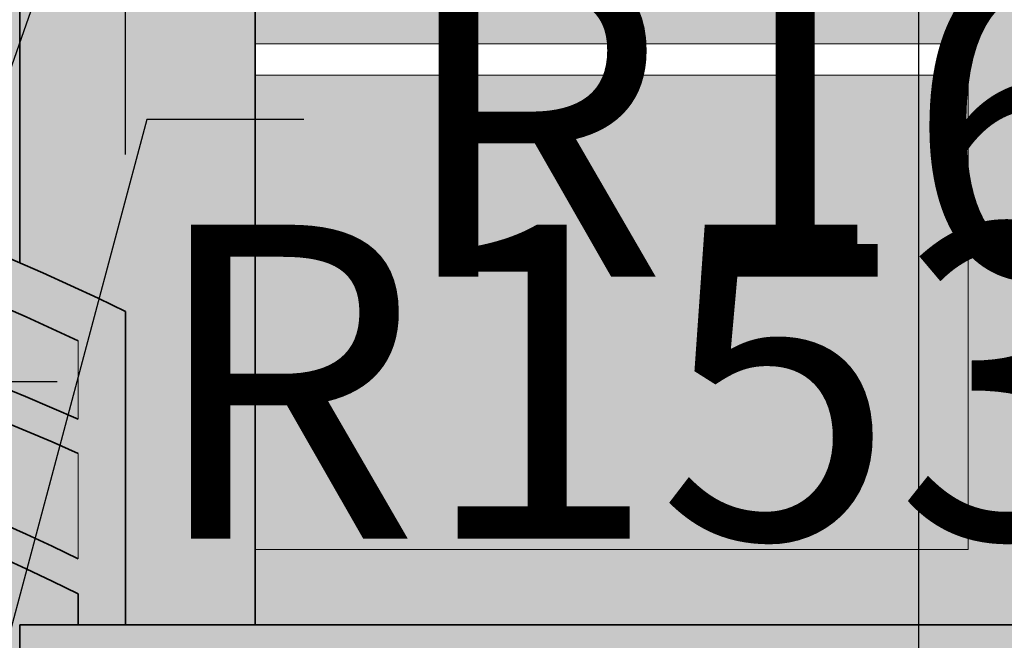
# Model space of a CAD drawing. Units: millimetres. Extents: x 130 to 1021, y 147 to 699.
# Tile 32 of 40: x 487 to 550, y 476 to 515. Entities that reach past the tile are written whole.
import ezdxf

# ---------------------------------------------------------------- set-up
doc = ezdxf.new("R2010")
doc.units = ezdxf.units.MM
doc.header["$MEASUREMENT"] = 0
for name, color, linetype, lineweight in [('A-ANNO-DIMS', 2, 'Continuous', 18), ('A-ELEV', 7, 'Continuous', 35), ('A-ELEV-PATT', 9, 'Continuous', 13), ('A-GLAZ', 4, 'Continuous', 18)]:
    doc.layers.add(name, color=color, linetype=linetype, lineweight=lineweight)
doc.styles.get("Standard").update_dxf_attribs({"font": 'arial.ttf'})
doc.dimstyles.get("Standard").update_dxf_attribs({"dimtxt": 20, "dimasz": 10, "dimexe": 10, "dimexo": 10, "dimgap": 5, "dimtad": 0, "dimtih": 1, "dimtoh": 1, "dimdec": 0, "dimzin": 0, "dimdsep": 46, "dimtxsty": 'Standard', "dimcen": 5, "dimadec": 0, "dimazin": 0, "dimtfac": 1, "dimtdec": 0, "dimtofl": 0, "dimtmove": 0, "dimatfit": 3, "dimfxl": 1, "dimtolj": 1, "dimtzin": 0, "dimarcsym": 0})

# ---------------------------------------------------------------- blocks, each defined once
blk = doc.blocks.new('*D11')
at = {"layer": 'A-ANNO-DIMS', "color": 0, "lineweight": -2, "transparency": 16777216}
for p, q in [((737.374, 648.699), (737.374, 149.739)), ((299.374, 566.947), (299.374, 149.739)), ((309.374, 159.739), (490.857, 159.739)), ((727.374, 159.739), (545.891, 159.739))]:
    blk.add_line(p, q, dxfattribs=at)
at = {"layer": 'A-ANNO-DIMS', "color": 0, "transparency": 16777216}
for points in [[(309.374, 161.406), (309.374, 158.073), (299.374, 159.739)], [(727.374, 161.406), (727.374, 158.073), (737.374, 159.739)]]:
    blk.add_solid(points, dxfattribs=at)
at = {"layer": 'Defpoints', "color": 0, "transparency": 16777216}
for p in [(737.374, 658.699), (299.374, 576.947), (737.374, 159.739)]:
    blk.add_point(p, dxfattribs=at)
at = {"layer": 'A-ANNO-DIMS', "color": 0, "transparency": 16777216, "insert": (518.374, 159.739), "char_height": 20, "attachment_point": 5}
blk.add_mtext('\\A1;438', dxfattribs=at)
blk = doc.blocks.new('*D12')
at = {"layer": 'A-ANNO-DIMS', "color": 0, "lineweight": -2, "transparency": 16777216}
for p, q in [((477.374, 661.947), (265.074, 661.947)), ((275.074, 651.947), (275.074, 438.205)), ((275.074, 194.039), (275.074, 407.782)), ((357.163, 184.039), (265.074, 184.039))]:
    blk.add_line(p, q, dxfattribs=at)
at = {"layer": 'A-ANNO-DIMS', "color": 0, "transparency": 16777216}
for points in [[(273.407, 651.947), (276.74, 651.947), (275.074, 661.947)], [(273.407, 194.039), (276.74, 194.039), (275.074, 184.039)]]:
    blk.add_solid(points, dxfattribs=at)
at = {"layer": 'Defpoints', "color": 0, "transparency": 16777216}
for p in [(275.074, 661.947), (487.374, 661.947), (367.163, 184.039)]:
    blk.add_point(p, dxfattribs=at)
at = {"layer": 'A-ANNO-DIMS', "color": 0, "transparency": 16777216, "insert": (275.074, 422.993), "char_height": 20, "attachment_point": 5}
blk.add_mtext('\\A1;477.9', dxfattribs=at)
blk = doc.blocks.new('*D19')
at = {"layer": 'A-ANNO-DIMS', "color": 0, "lineweight": -2, "transparency": 16777216}
for p, q in [((382.374, 388.947), (382.374, 696.247)), ((414.652, 510.881), (414.652, 696.247)), ((392.374, 686.247), (404.652, 686.247)), ((414.652, 686.247), (424.652, 686.247))]:
    blk.add_line(p, q, dxfattribs=at)
at = {"layer": 'A-ANNO-DIMS', "color": 0, "transparency": 16777216}
for points in [[(392.374, 687.914), (392.374, 684.581), (382.374, 686.247)], [(404.652, 687.914), (404.652, 684.581), (414.652, 686.247)]]:
    blk.add_solid(points, dxfattribs=at)
at = {"layer": 'Defpoints', "color": 0, "transparency": 16777216}
for p in [(414.652, 686.247), (414.652, 500.881), (382.374, 378.947)]:
    blk.add_point(p, dxfattribs=at)
at = {"layer": 'A-ANNO-DIMS', "color": 0, "transparency": 16777216, "insert": (463.411, 686.247), "char_height": 20, "attachment_point": 5}
blk.add_mtext('\\A1;32.28', dxfattribs=at)
blk = doc.blocks.new('*D20')
at = {"layer": 'A-ANNO-DIMS', "color": 0, "lineweight": -2, "transparency": 16777216}
for p, q in [((414.652, 510.881), (414.652, 696.247)), ((432.374, 388.947), (432.374, 696.247)), ((404.652, 686.247), (394.652, 686.247)), ((442.374, 686.247), (452.374, 686.247))]:
    blk.add_line(p, q, dxfattribs=at)
at = {"layer": 'A-ANNO-DIMS', "color": 0, "transparency": 16777216}
for points in [[(404.652, 687.914), (404.652, 684.581), (414.652, 686.247)], [(442.374, 687.914), (442.374, 684.581), (432.374, 686.247)]]:
    blk.add_solid(points, dxfattribs=at)
at = {"layer": 'Defpoints', "color": 0, "transparency": 16777216}
for p in [(432.374, 686.247), (414.652, 500.881), (432.374, 378.947)]:
    blk.add_point(p, dxfattribs=at)
at = {"layer": 'A-ANNO-DIMS', "color": 0, "transparency": 16777216, "insert": (490.075, 686.247), "char_height": 20, "attachment_point": 5}
blk.add_mtext('\\A1;17.72', dxfattribs=at)
blk = doc.blocks.new('*D21')
at = {"layer": 'A-ANNO-DIMS', "color": 0, "lineweight": -2, "transparency": 16777216}
for p, q in [((432.374, 388.947), (432.374, 696.247)), ((447.374, 656.947), (447.374, 696.247)), ((422.374, 686.247), (412.374, 686.247)), ((457.374, 686.247), (467.374, 686.247))]:
    blk.add_line(p, q, dxfattribs=at)
at = {"layer": 'A-ANNO-DIMS', "color": 0, "transparency": 16777216}
for points in [[(422.374, 687.914), (422.374, 684.581), (432.374, 686.247)], [(457.374, 687.914), (457.374, 684.581), (447.374, 686.247)]]:
    blk.add_solid(points, dxfattribs=at)
at = {"layer": 'Defpoints', "color": 0, "transparency": 16777216}
for p in [(447.374, 686.247), (447.374, 646.947), (432.374, 378.947)]:
    blk.add_point(p, dxfattribs=at)
at = {"layer": 'A-ANNO-DIMS', "color": 0, "transparency": 16777216, "insert": (485.832, 686.247), "char_height": 20, "attachment_point": 5}
blk.add_mtext('\\A1;15', dxfattribs=at)
blk = doc.blocks.new('*D22')
at = {"layer": 'A-ANNO-DIMS', "color": 0, "lineweight": -2, "transparency": 16777216}
for p, q in [((447.374, 656.947), (447.374, 696.247)), ((466.767, 403.947), (466.767, 696.247)), ((437.374, 686.247), (427.374, 686.247)), ((476.767, 686.247), (486.767, 686.247))]:
    blk.add_line(p, q, dxfattribs=at)
at = {"layer": 'A-ANNO-DIMS', "color": 0, "transparency": 16777216}
for points in [[(437.374, 687.914), (437.374, 684.581), (447.374, 686.247)], [(476.767, 687.914), (476.767, 684.581), (466.767, 686.247)]]:
    blk.add_solid(points, dxfattribs=at)
at = {"layer": 'Defpoints', "color": 0, "transparency": 16777216}
for p in [(466.767, 686.247), (447.374, 646.947), (466.767, 393.947)]:
    blk.add_point(p, dxfattribs=at)
at = {"layer": 'A-ANNO-DIMS', "color": 0, "transparency": 16777216, "insert": (532.34, 686.247), "char_height": 20, "attachment_point": 5}
blk.add_mtext('\\A1;19.393', dxfattribs=at)
blk = doc.blocks.new('*D23')
at = {"layer": 'A-ANNO-DIMS', "color": 0, "lineweight": -2, "transparency": 16777216}
for p, q in [((466.767, 403.947), (466.767, 696.247)), ((475.988, 209.039), (475.988, 696.247)), ((456.767, 686.247), (446.767, 686.247)), ((485.988, 686.247), (495.988, 686.247))]:
    blk.add_line(p, q, dxfattribs=at)
at = {"layer": 'A-ANNO-DIMS', "color": 0, "transparency": 16777216}
for points in [[(456.767, 687.914), (456.767, 684.581), (466.767, 686.247)], [(485.988, 687.914), (485.988, 684.581), (475.988, 686.247)]]:
    blk.add_solid(points, dxfattribs=at)
at = {"layer": 'Defpoints', "color": 0, "transparency": 16777216}
for p in [(475.988, 686.247), (466.767, 393.947), (475.988, 199.039)]:
    blk.add_point(p, dxfattribs=at)
at = {"layer": 'A-ANNO-DIMS', "color": 0, "transparency": 16777216, "insert": (534.631, 686.247), "char_height": 20, "attachment_point": 5}
blk.add_mtext('\\A1;9.222', dxfattribs=at)
blk = doc.blocks.new('*D24')
at = {"layer": 'A-ANNO-DIMS', "color": 0, "lineweight": -2, "transparency": 16777216}
for p, q in [((475.988, 209.039), (475.988, 696.247)), ((487.374, 671.947), (487.374, 696.247)), ((465.988, 686.247), (455.988, 686.247)), ((497.374, 686.247), (507.374, 686.247))]:
    blk.add_line(p, q, dxfattribs=at)
at = {"layer": 'A-ANNO-DIMS', "color": 0, "transparency": 16777216}
for points in [[(465.988, 687.914), (465.988, 684.581), (475.988, 686.247)], [(497.374, 687.914), (497.374, 684.581), (487.374, 686.247)]]:
    blk.add_solid(points, dxfattribs=at)
at = {"layer": 'Defpoints', "color": 0, "transparency": 16777216}
for p in [(487.374, 686.247), (487.374, 661.947), (475.988, 199.039)]:
    blk.add_point(p, dxfattribs=at)
at = {"layer": 'A-ANNO-DIMS', "color": 0, "transparency": 16777216, "insert": (553.022, 686.247), "char_height": 20, "attachment_point": 5}
blk.add_mtext('\\A1;11.385', dxfattribs=at)
blk = doc.blocks.new('*D25')
at = {"layer": 'A-ANNO-DIMS', "color": 0, "lineweight": -2, "transparency": 16777216}
for p, q in [((487.374, 671.947), (487.374, 696.247)), ((494.102, 506.908), (494.102, 696.247)), ((477.374, 686.247), (467.374, 686.247)), ((504.102, 686.247), (514.102, 686.247))]:
    blk.add_line(p, q, dxfattribs=at)
at = {"layer": 'A-ANNO-DIMS', "color": 0, "transparency": 16777216}
for points in [[(477.374, 687.914), (477.374, 684.581), (487.374, 686.247)], [(504.102, 687.914), (504.102, 684.581), (494.102, 686.247)]]:
    blk.add_solid(points, dxfattribs=at)
at = {"layer": 'Defpoints', "color": 0, "transparency": 16777216}
for p in [(494.102, 686.247), (487.374, 661.947), (494.102, 496.908)]:
    blk.add_point(p, dxfattribs=at)
at = {"layer": 'A-ANNO-DIMS', "color": 0, "transparency": 16777216, "insert": (552.922, 686.247), "char_height": 20, "attachment_point": 5}
blk.add_mtext('\\A1;6.728', dxfattribs=at)
blk = doc.blocks.new('*D26')
at = {"layer": 'A-ANNO-DIMS', "color": 0, "lineweight": -2, "transparency": 16777216}
for p, q in [((494.102, 506.908), (494.102, 696.247)), ((502.374, 593.947), (502.374, 696.247)), ((484.102, 686.247), (474.102, 686.247)), ((512.374, 686.247), (522.374, 686.247))]:
    blk.add_line(p, q, dxfattribs=at)
at = {"layer": 'A-ANNO-DIMS', "color": 0, "transparency": 16777216}
for points in [[(484.102, 687.914), (484.102, 684.581), (494.102, 686.247)], [(512.374, 687.914), (512.374, 684.581), (502.374, 686.247)]]:
    blk.add_solid(points, dxfattribs=at)
at = {"layer": 'Defpoints', "color": 0, "transparency": 16777216}
for p in [(502.374, 686.247), (502.374, 583.947), (494.102, 496.908)]:
    blk.add_point(p, dxfattribs=at)
at = {"layer": 'A-ANNO-DIMS', "color": 0, "transparency": 16777216, "insert": (561.03, 686.247), "char_height": 20, "attachment_point": 5}
blk.add_mtext('\\A1;8.272', dxfattribs=at)
blk = doc.blocks.new('*D27')
at = {"layer": 'A-ANNO-DIMS', "color": 0, "lineweight": -2, "transparency": 16777216}
for p, q in [((502.374, 593.947), (502.374, 696.247)), ((544.635, 396.264), (544.635, 696.247)), ((512.374, 686.247), (534.635, 686.247)), ((544.635, 686.247), (554.635, 686.247))]:
    blk.add_line(p, q, dxfattribs=at)
at = {"layer": 'A-ANNO-DIMS', "color": 0, "transparency": 16777216}
for points in [[(512.374, 687.914), (512.374, 684.581), (502.374, 686.247)], [(534.635, 687.914), (534.635, 684.581), (544.635, 686.247)]]:
    blk.add_solid(points, dxfattribs=at)
at = {"layer": 'Defpoints', "color": 0, "transparency": 16777216}
for p in [(544.635, 686.247), (502.374, 583.947), (544.635, 386.264)]:
    blk.add_point(p, dxfattribs=at)
at = {"layer": 'A-ANNO-DIMS', "color": 0, "transparency": 16777216, "insert": (593.776, 686.247), "char_height": 20, "attachment_point": 5}
blk.add_mtext('\\A1;42.26', dxfattribs=at)
blk = doc.blocks.new('*D28')
at = {"layer": 'A-ANNO-DIMS', "color": 0, "lineweight": -2, "transparency": 16777216}
for p, q in [((544.635, 396.264), (544.635, 696.247)), ((552.374, 593.947), (552.374, 696.247)), ((534.635, 686.247), (524.635, 686.247)), ((562.374, 686.247), (572.374, 686.247))]:
    blk.add_line(p, q, dxfattribs=at)
at = {"layer": 'A-ANNO-DIMS', "color": 0, "transparency": 16777216}
for points in [[(534.635, 687.914), (534.635, 684.581), (544.635, 686.247)], [(562.374, 687.914), (562.374, 684.581), (552.374, 686.247)]]:
    blk.add_solid(points, dxfattribs=at)
at = {"layer": 'Defpoints', "color": 0, "transparency": 16777216}
for p in [(552.374, 686.247), (552.374, 583.947), (544.635, 386.264)]:
    blk.add_point(p, dxfattribs=at)
at = {"layer": 'A-ANNO-DIMS', "color": 0, "transparency": 16777216, "insert": (611.057, 686.247), "char_height": 20, "attachment_point": 5}
blk.add_mtext('\\A1;7.738', dxfattribs=at)
blk = doc.blocks.new('*D54')
at = {"layer": 'A-ANNO-DIMS', "color": 0, "lineweight": -2, "transparency": 16777216}
for p, q in [((761.674, 473.947), (761.674, 483.947)), ((497.374, 463.947), (771.674, 463.947)), ((747.374, 403.69), (771.674, 403.69)), ((761.674, 393.69), (761.674, 383.69))]:
    blk.add_line(p, q, dxfattribs=at)
at = {"layer": 'A-ANNO-DIMS', "color": 0, "transparency": 16777216}
for points in [[(760.007, 473.947), (763.34, 473.947), (761.674, 463.947)], [(760.007, 393.69), (763.34, 393.69), (761.674, 403.69)]]:
    blk.add_solid(points, dxfattribs=at)
at = {"layer": 'Defpoints', "color": 0, "transparency": 16777216}
for p in [(487.374, 463.947), (761.674, 463.947), (737.374, 403.69)]:
    blk.add_point(p, dxfattribs=at)
at = {"layer": 'A-ANNO-DIMS', "color": 0, "transparency": 16777216, "insert": (761.674, 433.819), "char_height": 20, "attachment_point": 5}
blk.add_mtext('\\A1;60.26', dxfattribs=at)
blk = doc.blocks.new('*D55')
at = {"layer": 'A-ANNO-DIMS', "color": 0, "lineweight": -2, "transparency": 16777216}
for p, q in [((761.674, 486.947), (761.674, 496.947)), ((761.674, 496.947), (771.674, 496.947)), ((562.374, 476.947), (771.674, 476.947)), ((497.374, 463.947), (771.674, 463.947)), ((761.674, 453.947), (761.674, 443.947))]:
    blk.add_line(p, q, dxfattribs=at)
at = {"layer": 'A-ANNO-DIMS', "color": 0, "transparency": 16777216}
for points in [[(760.007, 486.947), (763.34, 486.947), (761.674, 476.947)], [(760.007, 453.947), (763.34, 453.947), (761.674, 463.947)]]:
    blk.add_solid(points, dxfattribs=at)
at = {"layer": 'Defpoints', "color": 0, "transparency": 16777216}
for p in [(552.374, 476.947), (761.674, 476.947), (487.374, 463.947)]:
    blk.add_point(p, dxfattribs=at)
at = {"layer": 'A-ANNO-DIMS', "color": 0, "transparency": 16777216, "insert": (790.057, 496.947), "char_height": 20, "attachment_point": 5}
blk.add_mtext('\\A1;13', dxfattribs=at)
blk = doc.blocks.new('*D65')
at = {"layer": 'A-ANNO-DIMS', "color": 0, "lineweight": -2, "transparency": 16777216}
for p, q in [((495.463, 509.127), (472.508, 423.108)), ((505.463, 509.127), (495.463, 509.127)), ((427.374, 248.979), (427.374, 258.979)), ((422.374, 253.979), (432.374, 253.979))]:
    blk.add_line(p, q, dxfattribs=at)
at = {"layer": 'A-ANNO-DIMS', "color": 0, "transparency": 16777216}
blk.add_solid([(470.898, 423.538), (474.118, 422.679), (469.93, 413.447)], dxfattribs=at)
at = {"layer": 'Defpoints', "color": 0, "transparency": 16777216}
for p in [(469.93, 413.447), (427.374, 253.979)]:
    blk.add_point(p, dxfattribs=at)
at = {"layer": 'A-ANNO-DIMS', "color": 0, "transparency": 16777216, "insert": (561.623, 509.127), "char_height": 20, "attachment_point": 5}
blk.add_mtext('\\A1;R165.05', dxfattribs=at)
blk = doc.blocks.new('*D67')
at = {"layer": 'A-ANNO-DIMS', "color": 0, "lineweight": -2, "transparency": 16777216}
for p, q in [((479.756, 492.431), (462.144, 412.223)), ((489.756, 492.431), (479.756, 492.431)), ((427.07, 247.496), (427.07, 257.496)), ((422.07, 252.496), (432.07, 252.496))]:
    blk.add_line(p, q, dxfattribs=at)
at = {"layer": 'A-ANNO-DIMS', "color": 0, "transparency": 16777216}
blk.add_solid([(460.516, 412.58), (463.772, 411.865), (459.999, 402.455)], dxfattribs=at)
at = {"layer": 'Defpoints', "color": 0, "transparency": 16777216}
for p in [(459.999, 402.455), (427.07, 252.496)]:
    blk.add_point(p, dxfattribs=at)
at = {"layer": 'A-ANNO-DIMS', "color": 0, "transparency": 16777216, "insert": (545.841, 492.431), "char_height": 20, "attachment_point": 5}
blk.add_mtext('\\A1;R153.53', dxfattribs=at)
blk = doc.blocks.new('*D69')
at = {"layer": 'A-ANNO-DIMS', "color": 0, "lineweight": -2, "transparency": 16777216}
for p, q in [((507.746, 572.261), (483.091, 501.813)), ((517.746, 572.261), (507.746, 572.261)), ((433.191, 354.23), (433.191, 364.23)), ((428.191, 359.23), (438.191, 359.23))]:
    blk.add_line(p, q, dxfattribs=at)
at = {"layer": 'A-ANNO-DIMS', "color": 0, "transparency": 16777216}
blk.add_solid([(481.518, 502.363), (484.664, 501.262), (479.788, 492.374)], dxfattribs=at)
at = {"layer": 'Defpoints', "color": 0, "transparency": 16777216}
for p in [(479.788, 492.374), (433.191, 359.23)]:
    blk.add_point(p, dxfattribs=at)
at = {"layer": 'A-ANNO-DIMS', "color": 0, "transparency": 16777216, "insert": (573.824, 572.261), "char_height": 20, "attachment_point": 5}
blk.add_mtext('\\A1;R141.06', dxfattribs=at)
blk = doc.blocks.new('*D71')
at = {"layer": 'A-ANNO-DIMS', "color": 0, "lineweight": -2, "transparency": 16777216}
for p, q in [((492.108, 581.609), (472.542, 512.666)), ((502.108, 581.609), (492.108, 581.609)), ((432.65, 367.109), (432.65, 377.109)), ((427.65, 372.109), (437.65, 372.109))]:
    blk.add_line(p, q, dxfattribs=at)
at = {"layer": 'A-ANNO-DIMS', "color": 0, "transparency": 16777216}
blk.add_solid([(470.938, 513.121), (474.145, 512.211), (469.812, 503.046)], dxfattribs=at)
at = {"layer": 'Defpoints', "color": 0, "transparency": 16777216}
for p in [(469.812, 503.046), (432.65, 372.109)]:
    blk.add_point(p, dxfattribs=at)
at = {"layer": 'A-ANNO-DIMS', "color": 0, "transparency": 16777216, "insert": (548.493, 581.609), "char_height": 20, "attachment_point": 5}
blk.add_mtext('\\A1;R136.1', dxfattribs=at)
blk = doc.blocks.new('*D72')
at = {"layer": 'A-ANNO-DIMS', "color": 0, "lineweight": -2, "transparency": 16777216}
for p, q in [((460.658, 573.64), (451.279, 503.49)), ((470.658, 573.64), (460.658, 573.64)), ((432.115, 355.142), (432.115, 365.142)), ((427.115, 360.142), (437.115, 360.142))]:
    blk.add_line(p, q, dxfattribs=at)
at = {"layer": 'A-ANNO-DIMS', "color": 0, "transparency": 16777216}
blk.add_solid([(449.628, 503.711), (452.931, 503.27), (449.954, 493.579)], dxfattribs=at)
at = {"layer": 'Defpoints', "color": 0, "transparency": 16777216}
for p in [(449.954, 493.579), (432.115, 360.142)]:
    blk.add_point(p, dxfattribs=at)
at = {"layer": 'A-ANNO-DIMS', "color": 0, "transparency": 16777216, "insert": (526.64, 573.64), "char_height": 20, "attachment_point": 5}
blk.add_mtext('\\A1;R134.62', dxfattribs=at)

msp = doc.modelspace()

# ---------------------------------------------------------------- hatches: boundary and pattern name
at = {"layer": 'A-ELEV-PATT'}
h = msp.add_hatch(color=256, dxfattribs=at)
h.dxf.hatch_style = 1
h.paths.add_polyline_path([(737.3738, 658.6988, 0.0135961), (632.4019, 661.9473), (607.3738, 661.9473), (487.3738, 661.9473), (487.3738, 649.9473), (607.3738, 649.9473), (632.3794, 649.9473, -0.0136841), (737.3738, 646.6784)])
h.paths.add_polyline_path([(732.3738, 643.9599, 0.0130529), (632.3738, 646.9473), (607.3738, 646.9473), (487.3738, 646.9473), (487.3738, 596.9473), (632.3738, 596.9473, -0.0130529), (732.3738, 593.9599)])
h.paths.add_polyline_path([(737.3738, 593.6732, 0.0137063), (632.3738, 596.9473), (487.3738, 596.9473), (487.3738, 586.9473), (632.355, 586.9473, -0.0137808), (737.3738, 583.6559)])
h.paths.add_polyline_path([(447.3738, 646.9473), (307.3738, 646.9473), (302.3738, 646.9473), (302.3738, 634.9473), (447.3738, 634.9473)])
h.paths.add_polyline_path([(447.3738, 631.9473), (307.3738, 631.9473), (307.3738, 586.9473), (447.3738, 586.9473)])
h.paths.add_polyline_path([(447.3738, 586.9473), (307.3738, 586.9473), (302.3738, 586.9473), (302.3738, 576.9473), (447.3738, 576.9473)])
h.paths.add_polyline_path([(447.3738, 573.9473), (367.3738, 573.9473), (367.3738, 539.9473), (447.3738, 539.9473)])
h.paths.add_polyline_path([(447.3738, 537.9473), (367.3738, 537.9473), (367.3738, 507.9473), (400.392, 507.4253, -0.001728), (401.3281, 507.6451, -0.5220025), (425.6117, 511.0391, -0.0391849), (447.3738, 510.4359), (447.3738, 510.7883)])
h.paths.add_polyline_path([(394.7238, 505.9473), (367.3738, 505.9473), (367.3738, 476.9473, -0.0146512), (375.8501, 480.2159), (376.1506, 499.2266, -0.0355419)])
h.paths.add_polyline_path([(632.3738, 583.9473), (552.3738, 583.9473), (552.3738, 550.9473), (632.3738, 550.9473)])
h.paths.add_polyline_path([(632.3738, 548.9473), (552.3738, 548.9473), (552.3738, 515.9473), (632.3738, 515.9473)])
h.paths.add_polyline_path([(632.3738, 513.9473), (552.3738, 513.9473), (552.3738, 476.9473), (632.3738, 476.9473)])
h.paths.add_polyline_path([(737.3738, 473.6903, 0.0136326), (632.3926, 476.9473), (552.3738, 476.9473), (487.3738, 476.9473), (487.3738, 466.9473), (632.3738, 466.9473, -0.0137063), (737.3738, 463.6732)])
h.paths.add_polyline_path([(732.3738, 460.9552, 0.0130741), (632.3681, 463.9473), (487.3738, 463.9473), (487.3738, 407.735, -0.0032286), (489.3544, 406.9473), (632.3926, 406.9473, -0.0129826), (732.3738, 403.9755)])
h.paths.add_polyline_path([(487.3738, 463.9473, 0.20133), (367.3738, 463.9473), (367.3738, 407.735, -0.1882031), (487.3738, 407.735)])
h.paths.add_polyline_path([(367.3738, 476.9473), (367.3738, 466.9473, -0.2013309), (487.3738, 466.9473), (487.3738, 476.9473, 0.20133)])
h.paths.add_polyline_path([(367.3738, 463.9473), (307.3738, 463.9473), (307.3738, 401.9473), (357.9413, 401.9473), (367.3738, 407.735)])
h.paths.add_polyline_path([(367.3738, 476.9473), (302.3738, 476.9473), (302.3738, 466.9473), (367.3738, 466.9473)])
h.paths.add_polyline_path([(632.8184, 366.9453), (552.3738, 366.9453), (552.3738, 393.9473), (632.8184, 393.9473)])
h.paths.add_polyline_path([(632.8184, 357.2114), (632.8184, 363.9453), (552.3738, 363.9453), (552.3738, 357.2114), (552.3738, 336.9453), (632.8184, 336.9453)])
h.paths.add_polyline_path([(632.8184, 333.9453), (552.3738, 333.9453), (552.3738, 306.9453), (632.8184, 306.9453)])
h.paths.add_polyline_path([(632.8184, 303.9453), (552.3738, 303.9453), (552.3738, 273.9473), (632.355, 273.9473, 0.0000608), (632.8184, 273.9491)])
h.paths.add_polyline_path([(737.3738, 403.6903, 0.0136326), (632.3926, 406.9473), (489.3544, 406.9473, 0.1915481), (367.3738, 407.735), (367.3738, 396.9473, -0.2013309), (487.3738, 396.9473), (632.3738, 396.9473, -0.0137063), (737.3738, 393.6732)])
h.paths.add_polyline_path([(357.9413, 401.9473), (307.3738, 401.9473), (307.3738, 391.9473), (357.9413, 391.9473)])
h.paths.add_polyline_path([(357.9413, 357.2114), (357.9413, 388.9473), (307.3738, 388.9473), (307.3738, 357.2114), (307.3738, 273.9473), (357.9413, 273.9473)])
h.paths.add_polyline_path([(732.3738, 263.93, -0.0130317), (632.3794, 260.9473), (466.7667, 260.9473), (466.7667, 240.9473), (469.8406, 236.978), (469.8406, 221.978), (472.9145, 218.0087), (472.9145, 213.9473), (607.3738, 213.9473), (732.3738, 213.9473)])
h.paths.add_polyline_path([(732.3738, 290.889), (722.479, 290.889), (722.479, 301.889), (732.3738, 301.889), (732.3738, 305.889), (722.479, 305.889), (722.479, 316.889), (732.3738, 316.889), (732.3738, 320.889), (722.479, 320.889), (722.479, 331.889), (732.3738, 331.889), (732.3738, 335.889), (722.479, 335.889), (722.479, 346.889), (732.3738, 346.889), (732.3738, 350.889), (722.479, 350.889), (722.479, 361.889), (732.3738, 361.889), (732.3738, 365.889), (722.479, 365.889), (722.479, 376.889), (732.3738, 376.889), (732.3738, 380.889), (722.479, 380.889), (722.479, 391.4848, 0.0005233), (718.479, 391.6843), (718.479, 380.889), (707.479, 380.889), (707.479, 392.1896, 0.0005231), (703.479, 392.3576), (703.479, 380.889), (692.479, 380.889), (692.479, 392.7765, 0.0005229), (688.479, 392.9131), (688.479, 380.889), (677.479, 380.889), (677.479, 393.2456, 0.0005228), (673.479, 393.3508), (673.479, 380.889), (662.479, 380.889), (662.479, 393.597, 0.0005227), (658.479, 393.6709), (658.479, 380.889), (647.479, 380.889), (647.479, 393.8308, 0.0005226), (643.479, 393.8732), (643.479, 380.889), (632.8184, 380.889), (632.8184, 376.889), (643.479, 376.889), (643.479, 365.889), (632.8184, 365.889), (632.8184, 361.889), (643.479, 361.889), (643.479, 350.889), (632.8184, 350.889), (632.8184, 346.889), (643.479, 346.889), (643.479, 335.889), (632.8184, 335.889), (632.8184, 331.889), (643.479, 331.889), (643.479, 320.889), (632.8184, 320.889), (632.8184, 316.889), (643.479, 316.889), (643.479, 305.889), (632.8184, 305.889), (632.8184, 301.889), (643.479, 301.889), (643.479, 290.889), (632.8184, 290.889), (632.8184, 286.889), (643.479, 286.889), (643.479, 274.0217, 0.0005246), (647.479, 274.0643), (647.479, 286.889), (658.479, 286.889), (658.479, 274.2248, 0.0005246), (662.479, 274.2989), (662.479, 286.889), (673.479, 286.889), (673.479, 274.546, 0.0005247), (677.479, 274.6516), (677.479, 286.889), (688.479, 286.889), (688.479, 274.9853, 0.0005248), (692.479, 275.1224), (692.479, 286.889), (703.479, 286.889), (703.479, 275.5429, 0.000525), (707.479, 275.7115), (707.479, 286.889), (718.479, 286.889), (718.479, 276.2187, 0.0005252), (722.479, 276.4189), (722.479, 286.889), (732.3738, 286.889)])
h.paths.add_polyline_path([(718.479, 290.889), (707.479, 290.889), (707.479, 301.889), (718.479, 301.889)], flags=16)
h.paths.add_polyline_path([(703.479, 290.889), (692.479, 290.889), (692.479, 301.889), (703.479, 301.889)], flags=16)
h.paths.add_polyline_path([(718.479, 305.889), (707.479, 305.889), (707.479, 316.889), (718.479, 316.889)], flags=16)
h.paths.add_polyline_path([(703.479, 305.889), (692.479, 305.889), (692.479, 316.889), (703.479, 316.889)], flags=16)
h.paths.add_polyline_path([(688.479, 290.889), (677.479, 290.889), (677.479, 301.889), (688.479, 301.889)], flags=16)
h.paths.add_polyline_path([(718.479, 320.889), (707.479, 320.889), (707.479, 331.889), (718.479, 331.889)], flags=16)
h.paths.add_polyline_path([(688.479, 305.889), (677.479, 305.889), (677.479, 316.889), (688.479, 316.889)], flags=16)
h.paths.add_polyline_path([(703.479, 320.889), (692.479, 320.889), (692.479, 331.889), (703.479, 331.889)], flags=16)
h.paths.add_polyline_path([(688.479, 320.889), (677.479, 320.889), (677.479, 331.889), (688.479, 331.889)], flags=16)
h.paths.add_polyline_path([(673.479, 290.889), (662.479, 290.889), (662.479, 301.889), (673.479, 301.889)], flags=16)
h.paths.add_polyline_path([(718.479, 335.889), (707.479, 335.889), (707.479, 346.889), (718.479, 346.889)], flags=16)
h.paths.add_polyline_path([(673.479, 305.889), (662.479, 305.889), (662.479, 316.889), (673.479, 316.889)], flags=16)
h.paths.add_polyline_path([(703.479, 335.889), (692.479, 335.889), (692.479, 346.889), (703.479, 346.889)], flags=16)
h.paths.add_polyline_path([(673.479, 320.889), (662.479, 320.889), (662.479, 331.889), (673.479, 331.889)], flags=16)
h.paths.add_polyline_path([(688.479, 335.889), (677.479, 335.889), (677.479, 346.889), (688.479, 346.889)], flags=16)
h.paths.add_polyline_path([(658.479, 290.889), (647.479, 290.889), (647.479, 301.889), (658.479, 301.889)], flags=16)
h.paths.add_polyline_path([(718.479, 350.889), (707.479, 350.889), (707.479, 361.889), (718.479, 361.889)], flags=16)
h.paths.add_polyline_path([(658.479, 305.889), (647.479, 305.889), (647.479, 316.889), (658.479, 316.889)], flags=16)
h.paths.add_polyline_path([(703.479, 350.889), (692.479, 350.889), (692.479, 361.889), (703.479, 361.889)], flags=16)
h.paths.add_polyline_path([(673.479, 335.889), (662.479, 335.889), (662.479, 346.889), (673.479, 346.889)], flags=16)
h.paths.add_polyline_path([(658.479, 320.889), (647.479, 320.889), (647.479, 331.889), (658.479, 331.889)], flags=16)
h.paths.add_polyline_path([(688.479, 350.889), (677.479, 350.889), (677.479, 361.889), (688.479, 361.889)], flags=16)
h.paths.add_polyline_path([(718.479, 365.889), (707.479, 365.889), (707.479, 376.889), (718.479, 376.889)], flags=16)
h.paths.add_polyline_path([(658.479, 335.889), (647.479, 335.889), (647.479, 346.889), (658.479, 346.889)], flags=16)
h.paths.add_polyline_path([(673.479, 350.889), (662.479, 350.889), (662.479, 361.889), (673.479, 361.889)], flags=16)
h.paths.add_polyline_path([(703.479, 365.889), (692.479, 365.889), (692.479, 376.889), (703.479, 376.889)], flags=16)
h.paths.add_polyline_path([(688.479, 365.889), (677.479, 365.889), (677.479, 376.889), (688.479, 376.889)], flags=16)
h.paths.add_polyline_path([(658.479, 350.889), (647.479, 350.889), (647.479, 361.889), (658.479, 361.889)], flags=16)
h.paths.add_polyline_path([(673.479, 365.889), (662.479, 365.889), (662.479, 376.889), (673.479, 376.889)], flags=16)
h.paths.add_polyline_path([(658.479, 365.889), (647.479, 365.889), (647.479, 376.889), (658.479, 376.889)], flags=16)
h.paths.add_polyline_path([(732.3738, 503.9786), (722.3392, 503.9786), (722.3392, 514.9786), (732.3738, 514.9786), (732.3738, 518.9786), (722.3392, 518.9786), (722.3392, 529.9786), (732.3738, 529.9786), (732.3738, 533.9786), (722.3392, 533.9786), (722.3392, 544.9786), (732.3738, 544.9786), (732.3738, 546.9473), (732.3738, 548.9786), (722.3392, 548.9786), (722.3392, 559.9786), (732.3738, 559.9786), (732.3738, 563.9786), (722.3392, 563.9786), (722.3392, 574.9786), (732.3738, 574.9786), (732.3738, 578.9786), (722.3392, 578.9786), (722.3392, 581.4789, 0.000526), (718.3392, 581.6791), (718.3392, 578.9786), (707.3392, 578.9786), (707.3392, 582.1863, 0.0005258), (703.3392, 582.355), (703.3392, 578.9786), (692.3392, 578.9786), (692.3392, 582.7752, 0.0005257), (688.3392, 582.9123), (688.3392, 578.9786), (677.3392, 578.9786), (677.3392, 583.2457, 0.0005255), (673.3392, 583.3512), (673.3392, 578.9786), (662.3392, 578.9786), (662.3392, 583.5978, 0.0005254), (658.3392, 583.6718), (658.3392, 578.9786), (647.3392, 578.9786), (647.3392, 583.8317, 0.0005254), (643.3392, 583.8741), (643.3392, 578.9786), (632.3738, 578.9786), (632.3738, 574.9786), (643.3392, 574.9786), (643.3392, 563.9786), (632.3738, 563.9786), (632.3738, 559.9786), (643.3392, 559.9786), (643.3392, 548.9786), (632.3738, 548.9786), (632.3738, 544.9786), (643.3392, 544.9786), (643.3392, 533.9786), (632.3738, 533.9786), (632.3738, 529.9786), (643.3392, 529.9786), (643.3392, 518.9786), (632.3738, 518.9786), (632.3738, 515.9473), (632.3738, 514.9786), (643.3392, 514.9786), (643.3392, 503.9786), (632.3738, 503.9786), (632.3738, 499.9786), (643.3392, 499.9786), (643.3392, 488.9786), (632.3738, 488.9786), (632.3738, 484.9786), (643.3392, 484.9786), (643.3392, 476.8751, -0.0005191), (647.3392, 476.8332), (647.3392, 484.9786), (658.3392, 484.9786), (658.3392, 476.6752, -0.0005192), (662.3392, 476.6022), (662.3392, 484.9786), (673.3392, 484.9786), (673.3392, 476.3585, -0.0005193), (677.3392, 476.2543), (677.3392, 484.9786), (688.3392, 484.9786), (688.3392, 475.9248, -0.0005194), (692.3392, 475.7894), (692.3392, 484.9786), (703.3392, 484.9786), (703.3392, 475.3741, -0.0005195), (707.3392, 475.2075), (707.3392, 484.9786), (718.3392, 484.9786), (718.3392, 474.7064, -0.0005197), (722.3392, 474.5086), (722.3392, 484.9786), (732.3738, 484.9786), (732.3738, 488.9786), (722.3392, 488.9786), (722.3392, 499.9786), (732.3738, 499.9786)])
h.paths.add_polyline_path([(718.3392, 503.9786), (707.3392, 503.9786), (707.3392, 514.9786), (718.3392, 514.9786)], flags=16)
h.paths.add_polyline_path([(718.3392, 499.9786), (718.3392, 488.9786), (707.3392, 488.9786), (707.3392, 499.9786)], flags=16)
h.paths.add_polyline_path([(718.3392, 518.9786), (707.3392, 518.9786), (707.3392, 529.9786), (718.3392, 529.9786)], flags=16)
h.paths.add_polyline_path([(703.3392, 503.9786), (692.3392, 503.9786), (692.3392, 514.9786), (703.3392, 514.9786)], flags=16)
h.paths.add_polyline_path([(703.3392, 499.9786), (703.3392, 488.9786), (692.3392, 488.9786), (692.3392, 499.9786)], flags=16)
h.paths.add_polyline_path([(703.3392, 518.9786), (692.3392, 518.9786), (692.3392, 529.9786), (703.3392, 529.9786)], flags=16)
h.paths.add_polyline_path([(718.3392, 533.9786), (707.3392, 533.9786), (707.3392, 544.9786), (718.3392, 544.9786)], flags=16)
h.paths.add_polyline_path([(688.3392, 503.9786), (677.3392, 503.9786), (677.3392, 514.9786), (688.3392, 514.9786)], flags=16)
h.paths.add_polyline_path([(688.3392, 499.9786), (688.3392, 488.9786), (677.3392, 488.9786), (677.3392, 499.9786)], flags=16)
h.paths.add_polyline_path([(703.3392, 533.9786), (692.3392, 533.9786), (692.3392, 544.9786), (703.3392, 544.9786)], flags=16)
h.paths.add_polyline_path([(688.3392, 518.9786), (677.3392, 518.9786), (677.3392, 529.9786), (688.3392, 529.9786)], flags=16)
h.paths.add_polyline_path([(688.3392, 533.9786), (677.3392, 533.9786), (677.3392, 544.9786), (688.3392, 544.9786)], flags=16)
h.paths.add_polyline_path([(718.3392, 548.9786), (707.3392, 548.9786), (707.3392, 559.9786), (718.3392, 559.9786)], flags=16)
h.paths.add_polyline_path([(673.3392, 503.9786), (662.3392, 503.9786), (662.3392, 514.9786), (673.3392, 514.9786)], flags=16)
h.paths.add_polyline_path([(673.3392, 499.9786), (673.3392, 488.9786), (662.3392, 488.9786), (662.3392, 499.9786)], flags=16)
h.paths.add_polyline_path([(703.3392, 548.9786), (692.3392, 548.9786), (692.3392, 559.9786), (703.3392, 559.9786)], flags=16)
h.paths.add_polyline_path([(673.3392, 518.9786), (662.3392, 518.9786), (662.3392, 529.9786), (673.3392, 529.9786)], flags=16)
h.paths.add_polyline_path([(688.3392, 548.9786), (677.3392, 548.9786), (677.3392, 559.9786), (688.3392, 559.9786)], flags=16)
h.paths.add_polyline_path([(673.3392, 533.9786), (662.3392, 533.9786), (662.3392, 544.9786), (673.3392, 544.9786)], flags=16)
h.paths.add_polyline_path([(718.3392, 563.9786), (707.3392, 563.9786), (707.3392, 574.9786), (718.3392, 574.9786)], flags=16)
h.paths.add_polyline_path([(658.3392, 503.9786), (647.3392, 503.9786), (647.3392, 514.9786), (658.3392, 514.9786)], flags=16)
h.paths.add_polyline_path([(658.3392, 499.9786), (658.3392, 488.9786), (647.3392, 488.9786), (647.3392, 499.9786)], flags=16)
h.paths.add_polyline_path([(703.3392, 563.9786), (692.3392, 563.9786), (692.3392, 574.9786), (703.3392, 574.9786)], flags=16)
h.paths.add_polyline_path([(658.3392, 518.9786), (647.3392, 518.9786), (647.3392, 529.9786), (658.3392, 529.9786)], flags=16)
h.paths.add_polyline_path([(673.3392, 548.9786), (662.3392, 548.9786), (662.3392, 559.9786), (673.3392, 559.9786)], flags=16)
h.paths.add_polyline_path([(688.3392, 563.9786), (677.3392, 563.9786), (677.3392, 574.9786), (688.3392, 574.9786)], flags=16)
h.paths.add_polyline_path([(658.3392, 533.9786), (647.3392, 533.9786), (647.3392, 544.9786), (658.3392, 544.9786)], flags=16)
h.paths.add_polyline_path([(673.3392, 563.9786), (662.3392, 563.9786), (662.3392, 574.9786), (673.3392, 574.9786)], flags=16)
h.paths.add_polyline_path([(658.3392, 548.9786), (647.3392, 548.9786), (647.3392, 559.9786), (658.3392, 559.9786)], flags=16)
h.paths.add_polyline_path([(658.3392, 563.9786), (647.3392, 563.9786), (647.3392, 574.9786), (658.3392, 574.9786)], flags=16)
h = msp.add_hatch(color=256, dxfattribs=at)
h.dxf.hatch_style = 1
h.paths.add_polyline_path([(447.3738, 576.9473), (302.3738, 576.9473), (302.3738, 573.9473), (447.3738, 573.9473)])
h.paths.add_polyline_path([(487.3738, 583.9473), (487.3738, 586.9473), (447.3738, 576.9473), (447.3738, 573.9473)])
h.paths.add_polyline_path([(632.355, 586.9473), (487.3738, 586.9473), (487.3738, 583.9473), (632.3738, 583.9473), (632.3738, 583.9472, -0.0138), (737.3738, 580.6507), (737.3738, 583.6559, 0.0137808)])
h.paths.add_polyline_path([(367.3738, 466.9473), (302.3738, 466.9473), (302.3738, 463.9473), (367.3738, 463.9473)])
h.paths.add_polyline_path([(487.3738, 463.9473), (487.3738, 466.9473, 0.2013309), (367.3738, 466.9473), (367.3738, 463.9473, -0.20133)])
h.paths.add_polyline_path([(632.3738, 466.9473), (487.3738, 466.9473), (487.3738, 463.9473), (632.3681, 463.9473, -0.0137285), (737.3738, 460.6681), (737.3738, 463.6732, 0.0137063)])
h.paths.add_polyline_path([(632.3738, 396.9473), (487.3738, 396.9473, 0.2013309), (367.3738, 396.9473), (367.3738, 393.9473, -0.2023717), (486.7667, 393.9473), (632.3681, 393.9473, -0.0137285), (737.3738, 390.6681), (737.3738, 393.6732, 0.0137063)])
h.paths.add_polyline_path([(357.9413, 391.9473), (307.3738, 391.9473), (307.3738, 388.9473), (357.9413, 388.9473)])
h.paths.add_polyline_path([(367.3738, 393.9473), (367.3738, 396.9473), (357.9413, 391.924), (357.9413, 388.9473), (358.058, 388.9473)])
h.paths.add_polyline_path([(737.3738, 264.2162), (737.3738, 267.2214, -0.0137063), (632.3738, 263.9473), (463.7667, 263.9473), (466.7667, 260.9473), (632.3794, 260.9473, 0.0136841)])
h.paths.add_polyline_path([(463.7667, 263.9473), (447.3738, 263.9473), (450.3738, 260.9473), (466.7667, 260.9473)])
h.paths.add_polyline_path([(447.3738, 263.9473), (432.3738, 263.9473), (432.3738, 260.9473), (450.3738, 260.9473)])
h.paths.add_polyline_path([(382.3738, 263.9473), (357.9413, 263.9473), (357.9413, 260.9473), (382.3738, 260.9473)])
h.paths.add_polyline_path([(357.9413, 263.9473), (307.3738, 263.9473), (307.3738, 260.9473), (357.9413, 260.9473)])
h = msp.add_hatch(color=256, dxfattribs=at)
h.paths.add_polyline_path([(327.3738, 569.884), (327.3738, 573.9473), (307.3738, 573.9473), (307.3738, 476.9473), (327.3738, 476.9473), (327.3738, 480.95)])
h.paths.add_polyline_path([(486.7667, 386.2639), (486.7667, 393.9473), (466.7667, 393.9473), (466.7667, 357.2114), (466.7667, 311.9335, 0.0342703), (486.7667, 308.4637)])
h.paths.add_polyline_path([(486.7667, 308.4637, -0.0342703), (466.7667, 311.9335), (466.7667, 273.9473), (486.7667, 273.9473)])
h.paths.add_polyline_path([(389.3738, 351.5473), (396.7693, 351.5473, -0.007027), (393.8774, 354.5473), (389.3738, 354.5473), (389.3738, 359.5775, -0.0190302), (382.3738, 368.424), (382.3738, 249.5473), (432.3738, 249.5473), (432.3738, 325.067, -0.0057673), (429.3738, 326.709), (429.3738, 257.5473), (426.3738, 257.5473), (426.3738, 328.4428, -0.0059254), (423.3738, 330.272), (423.3738, 315.7473), (389.3738, 315.7473), (389.3738, 332.1473), (420.4552, 332.1473, -0.008951), (416.0768, 335.1473), (389.3738, 335.1473)])
h.paths.add_polyline_path([(389.3738, 312.7473), (423.3738, 312.7473), (423.3738, 296.3473), (389.3738, 296.3473)], flags=16)
h.paths.add_polyline_path([(389.3738, 293.3473), (423.3738, 293.3473), (423.3738, 276.9473), (389.3738, 276.9473)], flags=16)
h.paths.add_polyline_path([(389.3738, 273.9473), (423.3738, 273.9473), (423.3738, 257.5473), (389.3738, 257.5473)], flags=16)
h.paths.add_polyline_path([(432.3738, 378.9473), (382.3738, 378.9473), (382.3738, 368.424, 0.0190302), (389.3738, 359.5775), (389.3738, 370.9473), (423.3738, 370.9473), (423.3738, 354.5473), (393.8774, 354.5473, 0.007027), (396.7693, 351.5473), (423.3738, 351.5473), (423.3738, 335.1473), (416.0768, 335.1473, 0.008951), (420.4552, 332.1473), (423.3738, 332.1473), (423.3738, 330.272, 0.0059254), (426.3738, 328.4428), (426.3738, 370.9473), (429.3738, 370.9473), (429.3738, 326.709, 0.0057673), (432.3738, 325.067)])
h.paths.add_polyline_path([(466.7667, 357.2114), (466.7667, 393.9473), (447.3738, 393.9473), (447.3738, 357.2114), (447.3738, 318.1243, 0.0063261), (450.8779, 316.785), (450.8779, 331.5915), (463.5608, 331.5915), (463.5608, 312.7571, 0.005582), (466.7667, 311.9335)])
h.paths.add_polyline_path([(450.8779, 334.5915), (450.8779, 360.0915), (463.5608, 360.0915), (463.5608, 334.5915)], flags=16)
h.paths.add_polyline_path([(450.8779, 363.0915), (450.8779, 388.6449), (463.5608, 388.6449), (463.5608, 363.0915)], flags=16)
h.paths.add_polyline_path([(466.7667, 311.9335, -0.005582), (463.5608, 312.7571), (463.5608, 306.0915), (450.8779, 306.0915), (450.8779, 316.785, -0.0063261), (447.3738, 318.1243), (447.3738, 273.9473), (466.7667, 273.9473)])
h.paths.add_polyline_path([(450.8779, 303.0915), (463.5608, 303.0915), (463.5608, 277.5915), (450.8779, 277.5915)], flags=16)
h.paths.add_polyline_path([(552.3738, 357.2114), (552.3738, 393.9473), (486.7667, 393.9473), (486.7667, 386.2639), (544.6354, 386.2639), (544.6354, 280.6619), (486.7667, 280.6619), (486.7667, 273.9473), (552.3738, 273.9473)])
h.paths.add_polyline_path([(487.3738, 583.9473), (472.3738, 580.1973), (472.3738, 507.0765), (472.3738, 505.4251, -0.0056452), (475.3738, 504.4942), (475.3738, 506.3543), (475.3738, 511.9473), (484.3738, 511.9473), (484.3738, 503.8134), (484.3738, 501.2439, -0.0058357), (487.3738, 500.0015)])
h.paths.add_polyline_path([(484.3738, 578.0434), (484.3738, 548.9473), (475.3738, 548.9473), (475.3738, 575.7934)], flags=16)
h.paths.add_polyline_path([(484.3738, 546.9473), (484.3738, 513.9473), (475.3738, 513.9473), (475.3738, 518.7148), (475.3738, 546.9473)], flags=16)
for points in [[(502.3738, 583.9473), (487.3738, 583.9473), (487.3738, 500.0015, -0.0133113), (494.1023, 496.908), (494.1023, 476.9473), (502.3738, 476.9473)], [(502.3738, 583.9473), (502.3738, 577.3739), (547.7773, 577.3739), (547.7773, 481.7432), (502.3738, 481.7432), (502.3738, 476.9473), (552.3738, 476.9473), (552.3738, 583.9473)]]:
    msp.add_hatch(color=256, dxfattribs=at).paths.add_polyline_path(points)
h = msp.add_hatch(color=256, dxfattribs=at)
h.dxf.hatch_style = 1
h.paths.add_polyline_path([(364.0891, 218.0087), (361.0152, 221.978), (361.0152, 236.978), (357.9413, 240.9473), (357.9413, 195.9473), (367.163, 184.0395), (367.163, 199.0395), (364.0891, 203.0087)])
h.paths.add_polyline_path([(502.3738, 537.2685), (502.3738, 513.9473), (547.7773, 513.9473), (547.7773, 537.2685)])
h.paths.add_polyline_path([(502.3738, 511.9473), (502.3738, 481.7432), (547.7773, 481.7432), (547.7773, 511.9473)])
h.paths.add_polyline_path([(327.3738, 529.7), (327.3738, 509.9473), (363.922, 509.9473), (363.922, 529.7)])
h.paths.add_polyline_path([(327.3738, 507.9473), (327.3738, 480.95), (363.922, 480.95), (363.922, 507.9473)])
h = msp.add_hatch(color=256, dxfattribs=at)
h.paths.add_polyline_path([(375.8501, 480.2159, -0.0051389), (378.8667, 481.244), (378.8725, 481.6093, -0.2220519), (491.1023, 478.9257), (491.1023, 476.9473), (494.1023, 476.9473), (494.1023, 496.908, 0.2225165), (376.1506, 499.2266)])
h.paths.add_polyline_path([(379.1197, 497.2486, -0.2152592), (491.1023, 495.0271), (491.1023, 490.0474, 0.2040153), (379.0311, 491.6449)], flags=16)
h.paths.add_polyline_path([(491.1023, 487.8572), (491.1023, 481.1546, 0.1695534), (402.9637, 491.5717, -0.0927216), (400.3891, 496.4261, -0.1659296)], flags=16)
h = msp.add_hatch(color=256, dxfattribs=at)
h.paths.add_polyline_path([(475.3738, 493.8379, 0.0055529), (472.3738, 494.7416), (472.3738, 488.6052, -0.0058604), (475.3738, 487.6263)])
h.paths.add_polyline_path([(475.3738, 485.5124, 0.0059584), (472.3738, 486.5077), (472.3738, 482.3533, -0.0050707), (475.3738, 481.4101)])
h.paths.add_polyline_path([(491.1023, 478.9257, 0.0077884), (487.3738, 480.7054), (487.3738, 476.9473), (491.1023, 476.9473)])
h.paths.add_polyline_path([(487.3738, 480.7054, 0.0061864), (484.3738, 482.0358), (484.3738, 478.1696, -0.0052234), (487.3738, 476.9473)])
h.paths.add_polyline_path([(487.3738, 489.4717, 0.0057318), (484.3738, 490.6796), (484.3738, 484.2088, -0.0060769), (487.3738, 482.902)])
h.paths.add_polyline_path([(491.1023, 487.8572, 0.0072012), (487.3738, 489.4717), (487.3738, 482.902, -0.0076471), (491.1023, 481.1546)])
h.paths.add_polyline_path([(487.3738, 496.7317, 0.0059873), (484.3738, 498.0065), (484.3738, 492.8236, -0.005639), (487.3738, 491.6352)])
h.paths.add_polyline_path([(491.1023, 495.0271, 0.0075306), (487.3738, 496.7317), (487.3738, 491.6352, -0.0070821), (491.1023, 490.0474)])

# ---------------------------------------------------------------- linework, layer by layer
at = {"layer": 'A-ELEV'}
for p, q in [((487.3738, 500.0015), (487.3738, 646.9473)), ((502.3738, 583.9473), (502.3738, 476.9473)), ((494.1023, 476.9473), (494.1023, 496.908)), ((491.1023, 476.9473), (491.1023, 478.9257)), ((487.3738, 407.735), (487.3738, 476.9473)), ((632.3738, 476.9473), (487.3738, 476.9473))]:
    msp.add_line(p, q, dxfattribs=at)
for centre, radius, start, end in [((432.6505, 372.1087), 139.1086, 63.78413, 113.963624), ((432.6505, 372.1087), 136.1086, 64.567343, 113.15965), ((433.1906, 359.2304), 143.0624, 66.12141, 112.245303), ((433.1906, 359.2304), 141.0624, 65.761287, 112.593106), ((432.115, 360.1423), 134.6235, 64.013142, 113.246941), ((432.115, 360.1423), 132.6235, 63.591208, 113.669232)]:
    msp.add_arc(centre, radius, start, end, dxfattribs=at)
at = {"layer": 'A-GLAZ'}
for p, q in [((487.3738, 502.8382), (487.3738, 514.8577)), ((547.7773, 513.9473), (502.3738, 513.9473)), ((547.7773, 511.9473), (502.3738, 511.9473)), ((487.3738, 500.0015), (487.3738, 502.8382)), ((491.1023, 490.0474), (491.1023, 495.0271)), ((491.1023, 481.1546), (491.1023, 487.8572))]:
    msp.add_line(p, q, dxfattribs=at)
msp.add_lwpolyline([(502.3738, 481.7432), (547.7773, 481.7432), (547.7773, 577.3739), (502.3738, 577.3739)], dxfattribs=at)

# ---------------------------------------------------------------- dimensions: what is measured, and where the dimension line sits
at = {"layer": 'A-ANNO-DIMS'}
for base, p1, p2, override, picture, middle in [((414.6525, 686.2473), (382.3738, 378.9473), (414.6525, 500.8811), {"dimdec": 2, "dimlfac": 1, "dimrnd": 0, "dimzin": 0, "dimdsep": 46, "dimlunit": 2}, '*D19', (463.411, 686.2473)), ((432.3738, 686.2473), (414.6525, 500.8811), (432.3738, 378.9473), {"dimdec": 2, "dimlfac": 1, "dimrnd": 0, "dimzin": 0, "dimdsep": 46, "dimlunit": 2}, '*D20', (490.075, 686.2473)), ((447.3738, 686.2473), (432.3738, 378.9473), (447.3738, 646.9473), {"dimdec": 0, "dimlfac": 1, "dimrnd": 0, "dimzin": 0, "dimdsep": 46, "dimlunit": 2}, '*D21', (485.8322, 686.2473)), ((466.7667, 686.2473), (447.3738, 646.9473), (466.7667, 393.9473), {"dimdec": 3, "dimlfac": 1, "dimrnd": 0, "dimzin": 0, "dimdsep": 46, "dimlunit": 2}, '*D22', (532.3397, 686.2473)), ((475.9885, 686.2473), (466.7667, 393.9473), (475.9885, 199.0395), {"dimdec": 3, "dimlfac": 1, "dimrnd": 0, "dimzin": 0, "dimdsep": 46, "dimlunit": 2}, '*D23', (534.631, 686.2473)), ((487.3738, 686.2473), (475.9885, 199.0395), (487.3738, 661.9473), {"dimdec": 3, "dimlfac": 1, "dimrnd": 0, "dimzin": 0, "dimdsep": 46, "dimlunit": 2}, '*D24', (553.0218, 686.2473)), ((494.10227, 686.2473), (487.37378, 661.9473), (494.10227, 496.90803), {"dimdec": 3, "dimlfac": 1, "dimrnd": 0, "dimzin": 0, "dimdsep": 46, "dimlunit": 2}, '*D25', (552.92219, 686.2473)), ((502.37378, 686.2473), (494.10227, 496.90803), (502.37378, 583.9473), {"dimdec": 3, "dimlfac": 1, "dimrnd": 0, "dimzin": 0, "dimdsep": 46, "dimlunit": 2}, '*D26', (561.02999, 686.2473)), ((544.6354, 686.2473), (502.3738, 583.9473), (544.6354, 386.2639), {"dimdec": 2, "dimlfac": 1, "dimrnd": 0, "dimzin": 0, "dimdsep": 46, "dimlunit": 2}, '*D27', (593.776, 686.2473)), ((552.3738, 686.2473), (544.6354, 386.2639), (552.3738, 583.9473), {"dimdec": 3, "dimlfac": 1, "dimrnd": 0, "dimzin": 0, "dimdsep": 46, "dimlunit": 2}, '*D28', (611.0573, 686.2473)), ((737.3738, 159.7395), (299.3738, 576.9473), (737.3738, 658.6988), {"dimdec": 0, "dimlfac": 1, "dimrnd": 0, "dimzin": 0, "dimdsep": 46, "dimlunit": 2}, '*D11', (518.3738, 159.7395))]:
    dim = msp.add_linear_dim(base=base, p1=p1, p2=p2, dimstyle='Standard', override=override, dxfattribs=at)
    dim.commit()
    dim.dimension.update_dxf_attribs({"geometry": picture, "text_midpoint": middle})
for base, p1, p2, override, picture, middle in [((275.0738, 661.9473), (367.163, 184.0395), (487.3738, 661.9473), {"dimdec": 1, "dimlfac": 1, "dimrnd": 0, "dimzin": 0, "dimdsep": 46, "dimlunit": 2}, '*D12', (275.0738, 422.9934)), ((761.6738, 476.9473), (487.3738, 463.9473), (552.3738, 476.9473), {"dimdec": 0, "dimlfac": 1, "dimrnd": 0, "dimzin": 0, "dimdsep": 46, "dimlunit": 2}, '*D55', (790.0571, 496.9473)), ((761.6738, 463.9473), (737.3738, 403.6903), (487.3738, 463.9473), {"dimdec": 2, "dimlfac": 1, "dimrnd": 0, "dimzin": 0, "dimdsep": 46, "dimlunit": 2}, '*D54', (761.6738, 433.8188))]:
    dim = msp.add_linear_dim(base=base, p1=p1, p2=p2, angle=90, dimstyle='Standard', override=override, dxfattribs=at)
    dim.commit()
    dim.dimension.update_dxf_attribs({"geometry": picture, "text_midpoint": middle})
for center, mpoint, override, picture, middle in [((432.6505, 372.1087), (469.8116, 503.0461), {"dimdec": 1, "dimlfac": 1, "dimrnd": 0, "dimzin": 0, "dimdsep": 46, "dimlunit": 2}, '*D71', (548.493, 581.6085)), ((432.115, 360.1423), (449.9544, 493.5786), {"dimdec": 2, "dimlfac": 1, "dimrnd": 0, "dimzin": 0, "dimdsep": 46, "dimlunit": 2}, '*D72', (526.6403, 573.6404)), ((433.1906, 359.2304), (479.788, 492.3743), {"dimdec": 2, "dimlfac": 1, "dimrnd": 0, "dimzin": 0, "dimdsep": 46, "dimlunit": 2}, '*D69', (573.8242, 572.2606)), ((427.3738, 253.9788), (469.9297, 413.4465), {"dimdec": 2, "dimlfac": 1, "dimrnd": 0, "dimzin": 0, "dimdsep": 46, "dimlunit": 2}, '*D65', (561.6228, 509.1272)), ((427.0702, 252.4956), (459.999, 402.4554), {"dimdec": 2, "dimlfac": 1, "dimrnd": 0, "dimzin": 0, "dimdsep": 46, "dimlunit": 2}, '*D67', (545.8408, 492.4313))]:
    dim = msp.add_radius_dim(center=center, mpoint=mpoint, dimstyle='Standard', override=override, dxfattribs=at)
    dim.commit()
    dim.dimension.update_dxf_attribs({"geometry": picture, "text_midpoint": middle, "dimtype": 164})

doc.saveas('drawing.dxf')
